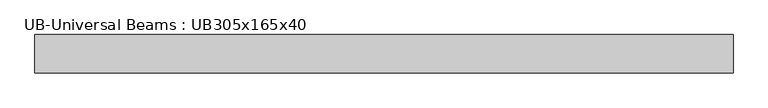
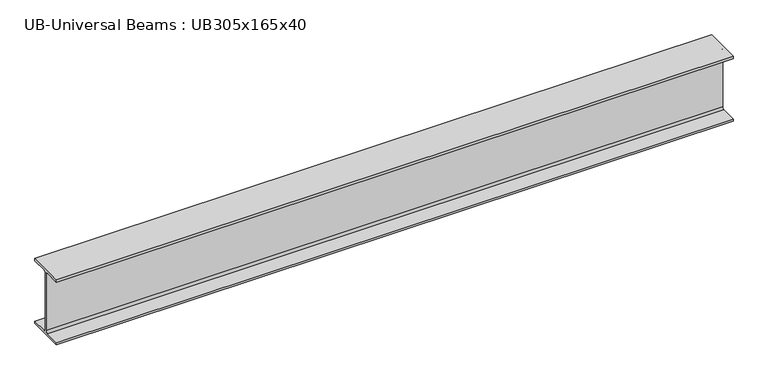
"""IFC4 building model written with IfcOpenShell, lengths in millimetres: beam geometry, UB-Universal Beams : UB305x165x40."""

from ifc_helpers import new_model, si_unit, point, frame, frame_2d, origin, place, context, project, spatial, polyline, circle_curve, trimmed, segment, composite_curve, outline, extrude, source, transform, mapped, element, save


def ub_universal_beams_ub305x165x40_f0dc7efd(model_context):
    return source(origin(), model_context, "Body", "SweptSolid", [
        extrude(outline(composite_curve([segment(polyline([(82.5, -141.5), (82.5, -151.7), (-82.5, -151.7), (-82.5, -141.5), (-11.9, -141.5)]), True, "CONTINUOUS"), segment(trimmed(circle_curve(frame_2d((-11.9, -132.6)), 8.9), [point((-11.9, -141.5))], [point((-3.0, -132.6))], True, "CARTESIAN"), True, "CONTINUOUS"), segment(polyline([(-3.0, -132.6), (-3.0, 132.6)]), True, "CONTINUOUS"), segment(trimmed(circle_curve(frame_2d((-11.9, 132.6)), 8.9), [point((-3.0, 132.6))], [point((-11.9, 141.5))], True, "CARTESIAN"), True, "CONTINUOUS"), segment(polyline([(-11.9, 141.5), (-82.5, 141.5), (-82.5, 151.7), (82.5, 151.7), (82.5, 141.5), (11.9, 141.5)]), True, "CONTINUOUS"), segment(trimmed(circle_curve(frame_2d((11.9, 132.6)), 8.9), [point((11.9, 141.5))], [point((3.0, 132.6))], True, "CARTESIAN"), True, "CONTINUOUS"), segment(polyline([(3.0, 132.6), (3.0, -132.6)]), True, "CONTINUOUS"), segment(trimmed(circle_curve(frame_2d((11.9, -132.6)), 8.9), [point((3.0, -132.6))], [point((11.9, -141.5))], True, "CARTESIAN"), True, "CONTINUOUS"), segment(polyline([(11.9, -141.5), (82.5, -141.5)]), True, "CONTINUOUS")], self_intersect=False)), frame((-1404.8, 0.0, 0.0), z_axis=(1.0, 0.0, 0.0), x_axis=(0.0, 1.0, 0.0)), (0.0, 0.0, 1.0), 2987.3),
    ])


if __name__ == "__main__":
    model = new_model("IFC4")
    model_context = context("Model", 3, world=origin())
    ifc_project = project(units=[si_unit("LENGTHUNIT", "METRE", prefix="MILLI")], contexts=[model_context])
    site = spatial("IfcSite", under=ifc_project)
    building = spatial("IfcBuilding", under=site)
    placement = place(None, origin())
    ub_universal_beams_ub305x165x40_shape = ub_universal_beams_ub305x165x40_f0dc7efd(model_context)
    element("IfcBeam", 1, ObjectType="UB-Universal Beams : UB305x165x40", at=placement, inside=building, context=model_context, shape_type="MappedRepresentation", body=[
        mapped(ub_universal_beams_ub305x165x40_shape, transform((0.0, 0.0, 0.0), x_axis=(1.0, 0.0, 0.0), y_axis=(0.0, 1.0, 0.0), z_axis=(0.0, 0.0, 1.0))),
    ])
    save(model, "model.ifc")

# Revit data of these elements
# Type "UB-Universal Beams : UB305x165x40"
#   Section Name Key = "UB305X165X40"
#   Width = 16.5 cm
#   Web Thickness = 0.6 cm
#   Web Fillet = 0.89 cm
#   Warping Constant = 164000.0 cm⁶
#   Torsional Moment of Inertia = 14.70 cm⁴
#   Section Area = 51.3 cm²
#   Plastic Modulus weak axis = 142.0 cm³
#   Plastic Modulus strong axis = 623.0 cm³
#   Nominal Weight = 40.2999 kgf/m
#   Moment of Inertia weak axis = 764.00 cm⁴
#   Moment of Inertia strong axis = 8503.00 cm⁴
#   Height = 30.34 cm
#   Flange Thickness = 1.02 cm
#   Elastic Modulus weak axis = 92.6 cm³
#   Elastic Modulus strong axis = 560.0 cm³
#   Centroid Vertical = 15.17 cm
#   Centroid Horizontal = 8.25 cm
#   Bolt Spacing = 9.0 cm
#   Length [instance default] = 1.5 m
#   Structural Material [instance default] = Metal - Steel 43-275
#   Type Comments = ""
#   Assembly Code = ""
# Element 1 (IfcBeam, "UB-Universal Beams : UB305x165x40")
#   Materials on its faces: "Metal - Steel 43-275"
# Materials
#   "Metal - Steel 43-275": class "Metal", colour RGB 247 247 247, transparency 0, Cost = 0
